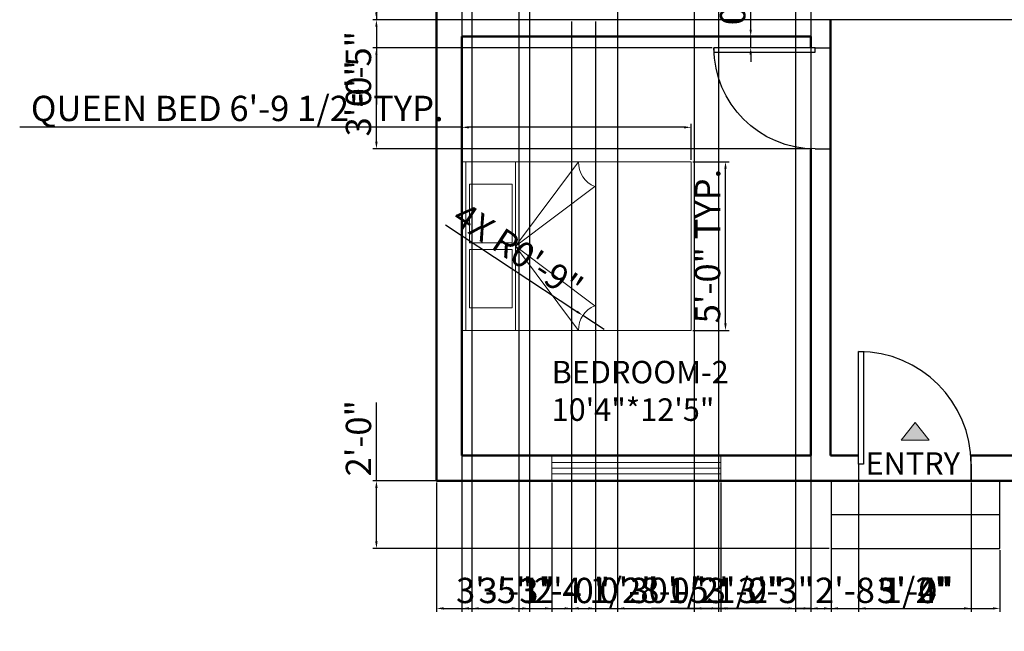
# Model space of a CAD drawing. Units: inches. Extents: x 2181 to 2717, y 1819 to 2296.
# Tile 1 of 5: x 2181 to 2531, y 1819 to 2036. Entities that reach past the tile are written whole.
import ezdxf

# ---------------------------------------------------------------- set-up
doc = ezdxf.new("R2010")
doc.units = ezdxf.units.IN
for name, color, linetype, lineweight in [('A-ANNO-DIMS', 2, 'Continuous', 13), ('A-ANNO-SYMB', 7, 'Continuous', 18), ('A-ANNO-SYMB-PATT', 7, 'Continuous', 18), ('A-ANNO-TEXT', 7, 'Continuous', 18), ('A-AREA-IDEN', 7, 'Continuous', 25), ('A-DOOR', 3, 'Continuous', 25), ('A-FLOR-STRS', 7, 'Continuous', 25), ('A-FURN', 8, 'Continuous', 18), ('A-GLAZ', 4, 'Continuous', 18), ('A-WALL', 7, 'Continuous', 50)]:
    doc.layers.add(name, color=color, linetype=linetype, lineweight=lineweight)
doc.styles.get("Standard").update_dxf_attribs({"font": 'arial.ttf'})
doc.dimstyles.new('ISO-25', dxfattribs={"dimtxt": 9, "dimasz": 2.5, "dimexe": 1.25, "dimexo": 0.625, "dimtad": 1, "dimlunit": 3, "dimtxsty": 'Standard', "dimcen": 2.5, "dimadec": 0, "dimazin": 0, "dimtfac": 1, "dimtmove": 0, "dimatfit": 3, "dimfxl": 1, "dimarcsym": 0})

# ---------------------------------------------------------------- blocks, each defined once
blk = doc.blocks.new('*U2')
for p, q in [((0, 0), (0, -6)), ((40, 0), (40, -6))]:
    blk.add_line(p, q)
blk.add_lwpolyline([(0, 0), (0, 40), (1.75, 40), (1.75, 0)], close=True)
blk.add_arc((0, 0), 40, 0, 90)
blk = doc.blocks.new('WIN-60IN')
for p, q in [((0, 0), (0, 9)), ((60, 0), (60, 9)), ((60, 6.5), (0, 6.5)), ((60, 4.5), (0, 4.5)), ((60, 2.5), (0, 2.5))]:
    blk.add_line(p, q)
blk = doc.blocks.new('BED-QUEEN-PLAN')
for p, q in [((60.01, 81.47), (0, 81.47)), ((0, 81.47), (0, 80)), ((60.01, 80), (60.01, 81.47)), ((0.01, 0), (0.01, 80)), ((0.01, 80), (60.01, 80)), ((8.01, 78.8), (28.81, 78.8)), ((8.01, 63.6), (8.01, 78.8)), ((28.81, 78.8), (28.81, 63.6)), ((31.21, 78.8), (52.01, 78.8)), ((31.21, 63.6), (31.21, 78.8)), ((52.01, 78.8), (52.01, 63.6)), ((60.01, 80), (60.01, 0)), ((28.81, 63.6), (8.01, 63.6)), ((52.01, 63.6), (31.21, 63.6)), ((60.01, 62.35), (0.01, 62.35)), ((30.01, 62.35), (0.01, 40)), ((8.81, 34.19), (30.01, 62.35)), ((30.01, 62.35), (60.01, 40)), ((51.22, 34.19), (30.01, 62.35)), ((60.01, 0), (0.01, 0))]:
    blk.add_line(p, q)
for centre, start, end in [((0.34, 30.93), 21.0875, 92.0428), ((59.69, 30.93), 87.9572, 158.9125)]:
    blk.add_arc(centre, 9.08, start, end)
blk = doc.blocks.new('*D19')
at = {"layer": 'A-ANNO-DIMS', "color": 0, "lineweight": -2, "transparency": 16777216}
for p, q in [((2338.35, 1997.93), (2181.23, 1997.93)), ((2338.35, 1986.33), (2338.35, 1999.18)), ((2417.32, 1997.93), (2340.85, 1997.93)), ((2419.82, 1986.33), (2419.82, 1999.18))]:
    blk.add_line(p, q, dxfattribs=at)
at = {"layer": 'A-ANNO-DIMS', "color": 0, "transparency": 16777216}
for points in [[(2340.85, 1998.34), (2340.85, 1997.51), (2338.35, 1997.93)], [(2417.32, 1998.34), (2417.32, 1997.51), (2419.82, 1997.93)]]:
    blk.add_solid(points, dxfattribs=at)
at = {"layer": 'Defpoints', "color": 0, "transparency": 16777216}
for p in [(2338.35, 1997.93), (2338.35, 1985.7), (2419.82, 1985.7)]:
    blk.add_point(p, dxfattribs=at)
at = {"layer": 'A-ANNO-DIMS', "color": 0, "transparency": 16777216, "insert": (2258.54, 2003.48), "char_height": 9, "attachment_point": 5}
blk.add_mtext('QUEEN BED 6\'-9 1/2" TYP.', dxfattribs=at)
blk = doc.blocks.new('*D20')
at = {"layer": 'A-ANNO-DIMS', "color": 0, "lineweight": -2, "transparency": 16777216}
for p, q in [((2420.44, 1985.7), (2433.29, 1985.7)), ((2432.04, 1928.19), (2432.04, 1983.2)), ((2420.44, 1925.69), (2433.29, 1925.69))]:
    blk.add_line(p, q, dxfattribs=at)
at = {"layer": 'A-ANNO-DIMS', "color": 0, "transparency": 16777216}
for points in [[(2431.62, 1983.2), (2432.46, 1983.2), (2432.04, 1985.7)], [(2431.62, 1928.19), (2432.46, 1928.19), (2432.04, 1925.69)]]:
    blk.add_solid(points, dxfattribs=at)
at = {"layer": 'Defpoints', "color": 0, "transparency": 16777216}
for p in [(2419.82, 1985.7), (2432.04, 1985.7), (2419.82, 1925.69)]:
    blk.add_point(p, dxfattribs=at)
at = {"layer": 'A-ANNO-DIMS', "color": 0, "transparency": 16777216, "insert": (2426.82, 1955.7), "char_height": 9, "attachment_point": 5, "rotation": 90}
blk.add_mtext('5\'-0" TYP.', dxfattribs=at)
blk = doc.blocks.new('*D34')
at = {"layer": 'A-ANNO-DIMS', "color": 0, "lineweight": -2, "transparency": 16777216}
for p, q in [((2329.35, 1871.58), (2329.35, 1825.6)), ((2370.35, 1871.58), (2370.35, 1825.6)), ((2331.85, 1826.85), (2367.85, 1826.85))]:
    blk.add_line(p, q, dxfattribs=at)
at = {"layer": 'A-ANNO-DIMS', "color": 0, "transparency": 16777216}
for points in [[(2331.85, 1827.27), (2331.85, 1826.44), (2329.35, 1826.85)], [(2367.85, 1827.27), (2367.85, 1826.44), (2370.35, 1826.85)]]:
    blk.add_solid(points, dxfattribs=at)
at = {"layer": 'Defpoints', "color": 0, "transparency": 16777216}
for p in [(2329.35, 1872.2), (2370.35, 1872.2), (2370.35, 1826.85)]:
    blk.add_point(p, dxfattribs=at)
at = {"layer": 'A-ANNO-DIMS', "color": 0, "transparency": 16777216, "insert": (2349.85, 1832.08), "char_height": 9, "attachment_point": 5}
blk.add_mtext('3\'-5"', dxfattribs=at)
blk = doc.blocks.new('*D35')
at = {"layer": 'A-ANNO-DIMS', "color": 0, "lineweight": -2, "transparency": 16777216}
for p, q in [((2430.35, 1871.58), (2430.35, 1825.6)), ((2469.56, 1871.58), (2469.56, 1825.6)), ((2432.85, 1826.85), (2467.06, 1826.85))]:
    blk.add_line(p, q, dxfattribs=at)
at = {"layer": 'A-ANNO-DIMS', "color": 0, "transparency": 16777216}
for points in [[(2432.85, 1827.27), (2432.85, 1826.44), (2430.35, 1826.85)], [(2467.06, 1827.27), (2467.06, 1826.44), (2469.56, 1826.85)]]:
    blk.add_solid(points, dxfattribs=at)
at = {"layer": 'Defpoints', "color": 0, "transparency": 16777216}
for p in [(2430.35, 1872.2), (2469.56, 1872.2), (2469.56, 1826.85)]:
    blk.add_point(p, dxfattribs=at)
at = {"layer": 'A-ANNO-DIMS', "color": 0, "transparency": 16777216, "insert": (2449.95, 1832.08), "char_height": 9, "attachment_point": 5}
blk.add_mtext('3\'-3"', dxfattribs=at)
blk = doc.blocks.new('*D36')
at = {"layer": 'A-ANNO-DIMS', "color": 0, "lineweight": -2, "transparency": 16777216}
for p, q in [((2479.35, 1871.58), (2479.35, 1825.6)), ((2519.35, 1871.58), (2519.35, 1825.6)), ((2481.85, 1826.85), (2516.85, 1826.85))]:
    blk.add_line(p, q, dxfattribs=at)
at = {"layer": 'A-ANNO-DIMS', "color": 0, "transparency": 16777216}
for points in [[(2481.85, 1827.27), (2481.85, 1826.44), (2479.35, 1826.85)], [(2516.85, 1827.27), (2516.85, 1826.44), (2519.35, 1826.85)]]:
    blk.add_solid(points, dxfattribs=at)
at = {"layer": 'Defpoints', "color": 0, "transparency": 16777216}
for p in [(2479.35, 1872.2), (2519.35, 1872.2), (2519.35, 1826.85)]:
    blk.add_point(p, dxfattribs=at)
at = {"layer": 'A-ANNO-DIMS', "color": 0, "transparency": 16777216, "insert": (2499.35, 1832.08), "char_height": 9, "attachment_point": 5}
blk.add_mtext('3\'-4"', dxfattribs=at)
blk = doc.blocks.new('*D37')
at = {"layer": 'A-ANNO-DIMS', "color": 0, "lineweight": -2, "transparency": 16777216}
for p, q in [((2469.56, 1847.58), (2469.56, 1825.6)), ((2529.56, 1847.58), (2529.56, 1825.6)), ((2472.06, 1826.85), (2527.06, 1826.85))]:
    blk.add_line(p, q, dxfattribs=at)
at = {"layer": 'A-ANNO-DIMS', "color": 0, "transparency": 16777216}
for points in [[(2472.06, 1827.27), (2472.06, 1826.44), (2469.56, 1826.85)], [(2527.06, 1827.27), (2527.06, 1826.44), (2529.56, 1826.85)]]:
    blk.add_solid(points, dxfattribs=at)
at = {"layer": 'Defpoints', "color": 0, "transparency": 16777216}
for p in [(2469.56, 1848.2), (2529.56, 1848.2), (2529.56, 1826.85)]:
    blk.add_point(p, dxfattribs=at)
at = {"layer": 'A-ANNO-DIMS', "color": 0, "transparency": 16777216, "insert": (2499.56, 1832.07), "char_height": 9, "attachment_point": 5}
blk.add_mtext('5\'-0"', dxfattribs=at)
blk = doc.blocks.new('*D38')
at = {"layer": 'A-ANNO-DIMS', "color": 0, "lineweight": -2, "transparency": 16777216}
for p, q in [((2308, 1872.2), (2308, 1900.03)), ((2468.93, 1872.2), (2306.75, 1872.2)), ((2308, 1850.7), (2308, 1869.7)), ((2468.93, 1848.2), (2306.75, 1848.2))]:
    blk.add_line(p, q, dxfattribs=at)
at = {"layer": 'A-ANNO-DIMS', "color": 0, "transparency": 16777216}
for points in [[(2307.58, 1869.7), (2308.41, 1869.7), (2308, 1872.2)], [(2307.58, 1850.7), (2308.41, 1850.7), (2308, 1848.2)]]:
    blk.add_solid(points, dxfattribs=at)
at = {"layer": 'Defpoints', "color": 0, "transparency": 16777216}
for p in [(2308, 1872.2), (2469.56, 1872.2), (2469.56, 1848.2)]:
    blk.add_point(p, dxfattribs=at)
at = {"layer": 'A-ANNO-DIMS', "color": 0, "transparency": 16777216, "insert": (2302.78, 1887.37), "char_height": 9, "attachment_point": 5, "rotation": 90}
blk.add_mtext('2\'-0"', dxfattribs=at)
blk = doc.blocks.new('*D41')
at = {"layer": 'A-ANNO-DIMS', "color": 0, "lineweight": -2, "transparency": 16777216}
for p, q in [((2338.35, 2119.58), (2338.35, 1825.6)), ((2362.35, 2119.58), (2362.35, 1825.6)), ((2340.85, 1826.85), (2359.85, 1826.85)), ((2362.35, 1826.85), (2390.17, 1826.85))]:
    blk.add_line(p, q, dxfattribs=at)
at = {"layer": 'A-ANNO-DIMS', "color": 0, "transparency": 16777216}
for points in [[(2340.85, 1827.27), (2340.85, 1826.44), (2338.35, 1826.85)], [(2359.85, 1827.27), (2359.85, 1826.44), (2362.35, 1826.85)]]:
    blk.add_solid(points, dxfattribs=at)
at = {"layer": 'Defpoints', "color": 0, "transparency": 16777216}
for p in [(2338.35, 2120.2), (2362.35, 2120.2), (2362.35, 1826.85)]:
    blk.add_point(p, dxfattribs=at)
at = {"layer": 'A-ANNO-DIMS', "color": 0, "transparency": 16777216, "insert": (2377.51, 1832.07), "char_height": 9, "attachment_point": 5}
blk.add_mtext('2\'-0"', dxfattribs=at)
blk = doc.blocks.new('*D43')
at = {"layer": 'A-ANNO-DIMS', "color": 0, "lineweight": -2, "transparency": 16777216}
for p, q in [((2393.61, 2225.64), (2393.61, 1825.6)), ((2429.61, 2225.64), (2429.61, 1825.6)), ((2396.11, 1826.85), (2427.11, 1826.85))]:
    blk.add_line(p, q, dxfattribs=at)
at = {"layer": 'A-ANNO-DIMS', "color": 0, "transparency": 16777216}
for points in [[(2396.11, 1827.27), (2396.11, 1826.44), (2393.61, 1826.85)], [(2427.11, 1827.27), (2427.11, 1826.44), (2429.61, 1826.85)]]:
    blk.add_solid(points, dxfattribs=at)
at = {"layer": 'Defpoints', "color": 0, "transparency": 16777216}
for p in [(2393.61, 2226.26), (2429.61, 2226.26), (2429.61, 1826.85)]:
    blk.add_point(p, dxfattribs=at)
at = {"layer": 'A-ANNO-DIMS', "color": 0, "transparency": 16777216, "insert": (2411.61, 1832.08), "char_height": 9, "attachment_point": 5}
blk.add_mtext('3\'-0"', dxfattribs=at)
blk = doc.blocks.new('*D45')
at = {"layer": 'A-ANNO-DIMS', "color": 0, "lineweight": -2, "transparency": 16777216}
for p, q in [((2429.61, 2225.64), (2429.61, 1825.6)), ((2462.35, 2222.58), (2462.35, 1825.6)), ((2432.11, 1826.85), (2459.85, 1826.85)), ((2462.35, 1826.85), (2511.15, 1826.85))]:
    blk.add_line(p, q, dxfattribs=at)
at = {"layer": 'A-ANNO-DIMS', "color": 0, "transparency": 16777216}
for points in [[(2432.11, 1827.27), (2432.11, 1826.44), (2429.61, 1826.85)], [(2459.85, 1827.27), (2459.85, 1826.44), (2462.35, 1826.85)]]:
    blk.add_solid(points, dxfattribs=at)
at = {"layer": 'Defpoints', "color": 0, "transparency": 16777216}
for p in [(2429.61, 2226.26), (2462.35, 2223.2), (2462.35, 1826.85)]:
    blk.add_point(p, dxfattribs=at)
at = {"layer": 'A-ANNO-DIMS', "color": 0, "transparency": 16777216, "insert": (2488, 1832.13), "char_height": 9, "attachment_point": 5}
blk.add_mtext('2\'-8 1/2"', dxfattribs=at)
blk = doc.blocks.new('*D47')
at = {"layer": 'A-ANNO-DIMS', "color": 0, "lineweight": -2, "transparency": 16777216}
for p, q in [((2341.86, 2155.89), (2341.86, 1825.6)), ((2358.61, 2155.89), (2358.61, 1825.6)), ((2344.36, 1826.85), (2356.11, 1826.85)), ((2358.61, 1826.85), (2406.41, 1826.85))]:
    blk.add_line(p, q, dxfattribs=at)
at = {"layer": 'A-ANNO-DIMS', "color": 0, "transparency": 16777216}
for points in [[(2344.36, 1827.27), (2344.36, 1826.44), (2341.86, 1826.85)], [(2356.11, 1827.27), (2356.11, 1826.44), (2358.61, 1826.85)]]:
    blk.add_solid(points, dxfattribs=at)
at = {"layer": 'Defpoints', "color": 0, "transparency": 16777216}
for p in [(2341.86, 2156.51), (2358.61, 2156.51), (2358.61, 1826.85)]:
    blk.add_point(p, dxfattribs=at)
at = {"layer": 'A-ANNO-DIMS', "color": 0, "transparency": 16777216, "insert": (2383.76, 1832.13), "char_height": 9, "attachment_point": 5}
blk.add_mtext('1\'-4 1/2"', dxfattribs=at)
blk = doc.blocks.new('*D53')
at = {"layer": 'A-ANNO-DIMS', "color": 0, "lineweight": -2, "transparency": 16777216}
for p, q in [((2308, 2043.69), (2308, 2046.19)), ((2549.72, 2041.19), (2306.75, 2041.19)), ((2308, 2041.19), (2308, 2036.2)), ((2549.72, 2036.2), (2306.75, 2036.2)), ((2308, 2033.7), (2308, 2006.03))]:
    blk.add_line(p, q, dxfattribs=at)
at = {"layer": 'A-ANNO-DIMS', "color": 0, "transparency": 16777216}
for points in [[(2307.58, 2043.69), (2308.41, 2043.69), (2308, 2041.19)], [(2307.58, 2033.7), (2308.41, 2033.7), (2308, 2036.2)]]:
    blk.add_solid(points, dxfattribs=at)
at = {"layer": 'Defpoints', "color": 0, "transparency": 16777216}
for p in [(2550.35, 2041.19), (2308, 2036.2), (2550.35, 2036.2)]:
    blk.add_point(p, dxfattribs=at)
at = {"layer": 'A-ANNO-DIMS', "color": 0, "transparency": 16777216, "insert": (2302.78, 2018.62), "char_height": 9, "attachment_point": 5, "rotation": 90}
blk.add_mtext('0\'-5"', dxfattribs=at)
blk = doc.blocks.new('*D54')
at = {"layer": 'A-ANNO-DIMS', "color": 0, "lineweight": -2, "transparency": 16777216}
for p, q in [((2377.35, 2035.58), (2377.35, 1825.6)), ((2385.85, 2035.58), (2385.85, 1825.6)), ((2379.85, 1826.85), (2383.35, 1826.85)), ((2385.85, 1826.85), (2434.49, 1826.85))]:
    blk.add_line(p, q, dxfattribs=at)
at = {"layer": 'A-ANNO-DIMS', "color": 0, "transparency": 16777216}
for points in [[(2379.85, 1827.27), (2379.85, 1826.44), (2377.35, 1826.85)], [(2383.35, 1827.27), (2383.35, 1826.44), (2385.85, 1826.85)]]:
    blk.add_solid(points, dxfattribs=at)
at = {"layer": 'Defpoints', "color": 0, "transparency": 16777216}
for p in [(2377.35, 2036.2), (2385.85, 2036.2), (2385.85, 1826.85)]:
    blk.add_point(p, dxfattribs=at)
at = {"layer": 'A-ANNO-DIMS', "color": 0, "transparency": 16777216, "insert": (2411.42, 1832.13), "char_height": 9, "attachment_point": 5}
blk.add_mtext('0\'-8 1/2"', dxfattribs=at)
blk = doc.blocks.new('*D55')
at = {"layer": 'A-ANNO-DIMS', "color": 0, "lineweight": -2, "transparency": 16777216}
for p, q in [((2338.35, 2035.58), (2338.35, 1825.6)), ((2377.35, 2035.58), (2377.35, 1825.6)), ((2340.85, 1826.85), (2374.85, 1826.85))]:
    blk.add_line(p, q, dxfattribs=at)
at = {"layer": 'A-ANNO-DIMS', "color": 0, "transparency": 16777216}
for points in [[(2340.85, 1827.27), (2340.85, 1826.44), (2338.35, 1826.85)], [(2374.85, 1827.27), (2374.85, 1826.44), (2377.35, 1826.85)]]:
    blk.add_solid(points, dxfattribs=at)
at = {"layer": 'Defpoints', "color": 0, "transparency": 16777216}
for p in [(2338.35, 2036.2), (2377.35, 2036.2), (2377.35, 1826.85)]:
    blk.add_point(p, dxfattribs=at)
at = {"layer": 'A-ANNO-DIMS', "color": 0, "transparency": 16777216, "insert": (2357.85, 1832.08), "char_height": 9, "attachment_point": 5}
blk.add_mtext('3\'-3"', dxfattribs=at)
blk = doc.blocks.new('*D56')
at = {"layer": 'A-ANNO-DIMS', "color": 0, "lineweight": -2, "transparency": 16777216}
for p, q in [((2549.72, 2114.2), (2306.75, 2114.2)), ((2308, 2038.7), (2308, 2111.7)), ((2549.72, 2036.2), (2306.75, 2036.2))]:
    blk.add_line(p, q, dxfattribs=at)
at = {"layer": 'A-ANNO-DIMS', "color": 0, "transparency": 16777216}
for points in [[(2307.58, 2111.7), (2308.41, 2111.7), (2308, 2114.2)], [(2307.58, 2038.7), (2308.41, 2038.7), (2308, 2036.2)]]:
    blk.add_solid(points, dxfattribs=at)
at = {"layer": 'Defpoints', "color": 0, "transparency": 16777216}
for p in [(2308, 2114.2), (2550.35, 2114.2), (2550.35, 2036.2)]:
    blk.add_point(p, dxfattribs=at)
at = {"layer": 'A-ANNO-DIMS', "color": 0, "transparency": 16777216, "insert": (2302.78, 2075.2), "char_height": 9, "attachment_point": 5, "rotation": 90}
blk.add_mtext('6\'-6"', dxfattribs=at)
blk = doc.blocks.new('*D57')
at = {"layer": 'A-ANNO-DIMS', "color": 0, "lineweight": -2, "transparency": 16777216}
for p, q in [((2456.94, 2119.58), (2456.94, 1825.6)), ((2462.35, 2119.58), (2462.35, 1825.6)), ((2454.44, 1826.85), (2405.8, 1826.85)), ((2462.35, 1826.85), (2456.94, 1826.85)), ((2464.85, 1826.85), (2467.35, 1826.85))]:
    blk.add_line(p, q, dxfattribs=at)
at = {"layer": 'A-ANNO-DIMS', "color": 0, "transparency": 16777216}
for points in [[(2454.44, 1827.27), (2454.44, 1826.44), (2456.94, 1826.85)], [(2464.85, 1827.27), (2464.85, 1826.44), (2462.35, 1826.85)]]:
    blk.add_solid(points, dxfattribs=at)
at = {"layer": 'Defpoints', "color": 0, "transparency": 16777216}
for p in [(2456.94, 2120.2), (2462.35, 2120.2), (2456.94, 1826.85)]:
    blk.add_point(p, dxfattribs=at)
at = {"layer": 'A-ANNO-DIMS', "color": 0, "transparency": 16777216, "insert": (2428.87, 1832.13), "char_height": 9, "attachment_point": 5}
blk.add_mtext('0\'-5 1/2"', dxfattribs=at)
blk = doc.blocks.new('*D58')
at = {"layer": 'A-ANNO-DIMS', "color": 0, "lineweight": -2, "transparency": 16777216}
for p, q in [((2420.94, 2119.58), (2420.94, 1825.6)), ((2456.94, 2119.58), (2456.94, 1825.6)), ((2423.44, 1826.85), (2454.44, 1826.85))]:
    blk.add_line(p, q, dxfattribs=at)
at = {"layer": 'A-ANNO-DIMS', "color": 0, "transparency": 16777216}
for points in [[(2423.44, 1827.27), (2423.44, 1826.44), (2420.94, 1826.85)], [(2454.44, 1827.27), (2454.44, 1826.44), (2456.94, 1826.85)]]:
    blk.add_solid(points, dxfattribs=at)
at = {"layer": 'Defpoints', "color": 0, "transparency": 16777216}
for p in [(2420.94, 2120.2), (2456.94, 2120.2), (2456.94, 1826.85)]:
    blk.add_point(p, dxfattribs=at)
at = {"layer": 'A-ANNO-DIMS', "color": 0, "transparency": 16777216, "insert": (2438.94, 1832.08), "char_height": 9, "attachment_point": 5}
blk.add_mtext('3\'-0"', dxfattribs=at)
blk = doc.blocks.new('*D59')
at = {"layer": 'A-ANNO-DIMS', "color": 0, "lineweight": -2, "transparency": 16777216}
for p, q in [((2427.32, 2026.24), (2306.75, 2026.24)), ((2308, 1992.78), (2308, 2023.74)), ((2461.72, 1990.28), (2306.75, 1990.28))]:
    blk.add_line(p, q, dxfattribs=at)
at = {"layer": 'A-ANNO-DIMS', "color": 0, "transparency": 16777216}
for points in [[(2307.58, 2023.74), (2308.41, 2023.74), (2308, 2026.24)], [(2307.58, 1992.78), (2308.41, 1992.78), (2308, 1990.28)]]:
    blk.add_solid(points, dxfattribs=at)
at = {"layer": 'Defpoints', "color": 0, "transparency": 16777216}
for p in [(2308, 2026.24), (2427.95, 2026.24), (2462.35, 1990.28)]:
    blk.add_point(p, dxfattribs=at)
at = {"layer": 'A-ANNO-DIMS', "color": 0, "transparency": 16777216, "insert": (2302.77, 2008.26), "char_height": 9, "attachment_point": 5, "rotation": 90}
blk.add_mtext('3\'-0"', dxfattribs=at)
blk = doc.blocks.new('*D60')
at = {"layer": 'A-ANNO-DIMS', "color": 0, "lineweight": -2, "transparency": 16777216}
for p, q in [((2441, 2032.7), (2441, 2060.38)), ((2461.72, 2030.2), (2439.75, 2030.2)), ((2441, 2026.24), (2441, 2030.2)), ((2461.72, 2026.24), (2439.75, 2026.24)), ((2441, 2023.74), (2441, 2021.24))]:
    blk.add_line(p, q, dxfattribs=at)
at = {"layer": 'A-ANNO-DIMS', "color": 0, "transparency": 16777216}
for points in [[(2440.58, 2032.7), (2441.41, 2032.7), (2441, 2030.2)], [(2440.58, 2023.74), (2441.41, 2023.74), (2441, 2026.24)]]:
    blk.add_solid(points, dxfattribs=at)
at = {"layer": 'Defpoints', "color": 0, "transparency": 16777216}
for p in [(2441, 2030.2), (2462.35, 2030.2), (2462.35, 2026.24)]:
    blk.add_point(p, dxfattribs=at)
at = {"layer": 'A-ANNO-DIMS', "color": 0, "transparency": 16777216, "insert": (2435.78, 2047.79), "char_height": 9, "attachment_point": 5, "rotation": 90}
blk.add_mtext('0\'-4"', dxfattribs=at)
blk = doc.blocks.new('*D62')
at = {"layer": 'A-ANNO-DIMS', "color": 0, "lineweight": -2, "transparency": 16777216}
for p, q in [((2332.51, 1963.26), (2379.23, 1932.41)), ((2388.89, 1926.03), (2381.32, 1931.03))]:
    blk.add_line(p, q, dxfattribs=at)
at = {"layer": 'A-ANNO-DIMS', "color": 0, "transparency": 16777216}
blk.add_solid([(2379.46, 1932.76), (2379, 1932.06), (2381.32, 1931.03)], dxfattribs=at)
at = {"layer": 'Defpoints', "color": 0, "transparency": 16777216}
for p in [(2381.32, 1931.03), (2388.89, 1926.03)]:
    blk.add_point(p, dxfattribs=at)
at = {"layer": 'A-ANNO-DIMS', "color": 0, "transparency": 16777216, "insert": (2357.7, 1952.88), "char_height": 9, "attachment_point": 5, "rotation": 326.565}
blk.add_mtext('4X R0\'-9"', dxfattribs=at)

msp = doc.modelspace()

# ---------------------------------------------------------------- hatches: boundary and pattern name
at = {"layer": 'A-ANNO-SYMB-PATT'}
h = msp.add_hatch(color=256, dxfattribs=at)
h.dxf.hatch_style = 1
h.paths.add_polyline_path([(2499.467, 1892.989), (2494.505, 1886.741), (2504.428, 1886.741)])

# ---------------------------------------------------------------- linework, layer by layer
at = {"layer": 'A-ANNO-SYMB'}
for p, q in [((2499.467, 1892.989), (2494.505, 1886.741)), ((2504.428, 1886.741), (2499.467, 1892.989)), ((2494.505, 1886.741), (2504.428, 1886.741))]:
    msp.add_line(p, q, dxfattribs=at)
at = {"layer": 'A-DOOR'}
msp.add_line((2519.346, 1872.205), (2519.346, 1881.205), dxfattribs=at)
at = {"layer": 'A-FLOR-STRS'}
for p, q in [((2469.556, 1872.205), (2469.556, 1848.205)), ((2529.556, 1848.205), (2529.556, 1872.205)), ((2469.556, 1860.205), (2529.556, 1860.205)), ((2469.556, 1848.205), (2517.556, 1848.205)), ((2517.556, 1848.205), (2529.556, 1848.205))]:
    msp.add_line(p, q, dxfattribs=at)
at = {"layer": 'A-WALL'}
for p, q in [((2329.346, 2256.205), (2329.346, 1872.205)), ((2469.346, 2036.205), (2469.346, 1881.205)), ((2338.346, 2030.205), (2462.346, 2030.205)), ((2338.346, 2030.205), (2338.346, 1881.205)), ((2462.346, 2030.205), (2462.346, 2026.245)), ((2462.346, 1990.28), (2462.346, 1881.205)), ((2338.346, 1881.205), (2462.346, 1881.205)), ((2469.346, 1881.205), (2479.346, 1881.205)), ((2519.346, 1881.205), (2620.346, 1881.205)), ((2329.346, 1872.205), (2629.346, 1872.205))]:
    msp.add_line(p, q, dxfattribs=at)

# ---------------------------------------------------------------- block references
at = {"layer": 'A-DOOR', "xscale": -0.9, "yscale": 0.9, "zscale": 0.9, "rotation": 90}
msp.add_blockref('*U2', (2463.946, 2026.245), dxfattribs=at)
at = {"layer": 'A-DOOR'}
msp.add_blockref('*U2', (2479.346, 1878.205), dxfattribs=at)
at = {"layer": 'A-FURN', "rotation": 90.00000000000033}
msp.add_blockref('BED-QUEEN-PLAN', (2419.819, 1925.692), dxfattribs=at)
at = {"layer": 'A-GLAZ'}
msp.add_blockref('WIN-60IN', (2370.346, 1872.205), dxfattribs=at)

# ---------------------------------------------------------------- texts
at = {"layer": 'A-ANNO-TEXT', "insert": (2481.794, 1882.39), "char_height": 8, "attachment_point": 1}
msp.add_mtext_dynamic_manual_height_columns('ENTRY', width=48.44663, gutter_width=12.5, heights=[0], dxfattribs=at)
at = {"layer": 'A-AREA-IDEN', "insert": (2370.243, 1914.883), "char_height": 8, "attachment_point": 1}
msp.add_mtext_dynamic_manual_height_columns('BEDROOM-2\\P10\'4"*12\'5"', width=59.66583, gutter_width=12.5, heights=[0], dxfattribs=at)

# ---------------------------------------------------------------- dimensions: what is measured, and where the dimension line sits
at = {"layer": 'A-ANNO-DIMS'}
for base, p1, p2, picture, middle in [((2429.61, 1826.855), (2393.61, 2226.263), (2429.61, 2226.263), '*D43', (2411.61, 1832.078)), ((2462.346, 1826.855), (2429.61, 2226.263), (2462.346, 2223.205), '*D45', (2487.996, 1832.133)), ((2358.609, 1826.855), (2341.861, 2156.51), (2358.609, 2156.51), '*D47', (2383.758, 1832.133)), ((2362.346, 1826.855), (2338.346, 2120.205), (2362.346, 2120.205), '*D41', (2377.51, 1832.075)), ((2456.942, 1826.855), (2462.346, 2120.205), (2456.942, 2120.205), '*D57', (2428.87, 1832.133)), ((2456.942, 1826.855), (2420.942, 2120.205), (2456.942, 2120.205), '*D58', (2438.942, 1832.078)), ((2377.346, 1826.855), (2338.346, 2036.205), (2377.346, 2036.205), '*D55', (2357.846, 1832.078)), ((2385.846, 1826.855), (2377.346, 2036.205), (2385.846, 2036.205), '*D54', (2411.419, 1832.133)), ((2370.346, 1826.855), (2329.346, 1872.205), (2370.346, 1872.205), '*D34', (2349.846, 1832.078)), ((2469.556, 1826.855), (2430.346, 1872.205), (2469.556, 1872.205), '*D35', (2449.951, 1832.078)), ((2519.346, 1826.855), (2479.346, 1872.205), (2519.346, 1872.205), '*D36', (2499.346, 1832.078)), ((2529.556, 1826.855), (2469.556, 1848.205), (2529.556, 1848.205), '*D37', (2499.556, 1832.075))]:
    dim = msp.add_linear_dim(base=base, p1=p1, p2=p2, dimstyle='ISO-25', override={"dimdec": 1, "dimlfac": 1, "dimrnd": 0, "dimzin": 1, "dimdsep": 46, "dimlunit": 4, "dimfrac": 2}, dxfattribs=at)
    dim.commit()
    dim.dimension.update_dxf_attribs({"geometry": picture, "text_midpoint": middle})
for base, p1, p2, picture, middle in [((2307.996, 2114.205), (2550.346, 2036.205), (2550.346, 2114.205), '*D56', (2302.776, 2075.205)), ((2440.996, 2030.205), (2462.346, 2026.245), (2462.346, 2030.205), '*D60', (2435.776, 2047.792)), ((2307.996, 2036.205), (2550.346, 2041.187), (2550.346, 2036.205), '*D53', (2302.776, 2018.617)), ((2307.996, 2026.245), (2462.346, 1990.28), (2427.946, 2026.245), '*D59', (2302.773, 2008.262)), ((2307.996, 1872.205), (2469.556, 1848.205), (2469.556, 1872.205), '*D38', (2302.776, 1887.368))]:
    dim = msp.add_linear_dim(base=base, p1=p1, p2=p2, angle=90, dimstyle='ISO-25', override={"dimdec": 1, "dimlfac": 1, "dimrnd": 0, "dimzin": 1, "dimdsep": 46, "dimlunit": 4, "dimfrac": 2}, dxfattribs=at)
    dim.commit()
    dim.dimension.update_dxf_attribs({"geometry": picture, "text_midpoint": middle})
for base, p1, p2, angle, text, picture, middle in [((2338.346, 1997.926), (2419.819, 1985.705), (2338.346, 1985.705), 180, 'QUEEN BED <> TYP.', '*D19', (2258.54, 2003.48)), ((2432.04, 1985.705), (2419.819, 1925.692), (2419.819, 1985.705), 90, '<> TYP.', '*D20', (2426.82, 1955.698))]:
    dim = msp.add_linear_dim(base=base, p1=p1, p2=p2, angle=angle, text=text, dimstyle='ISO-25', override={"dimdec": 1, "dimlfac": 1, "dimrnd": 0, "dimzin": 1, "dimdsep": 46, "dimlunit": 4, "dimfrac": 2}, dxfattribs=at)
    dim.commit()
    dim.dimension.update_dxf_attribs({"geometry": picture, "text_midpoint": middle})
dim = msp.add_radius_dim(center=(2388.892, 1926.028), mpoint=(2381.316, 1931.03), text='4X <>', dimstyle='ISO-25', override={"dimdec": 1, "dimlfac": 1, "dimrnd": 0, "dimzin": 1, "dimdsep": 46, "dimlunit": 4, "dimfrac": 2}, dxfattribs=at)
dim.commit()
dim.dimension.update_dxf_attribs({"geometry": '*D62', "text_midpoint": (2357.701, 1952.877)})

doc.saveas('drawing.dxf')
